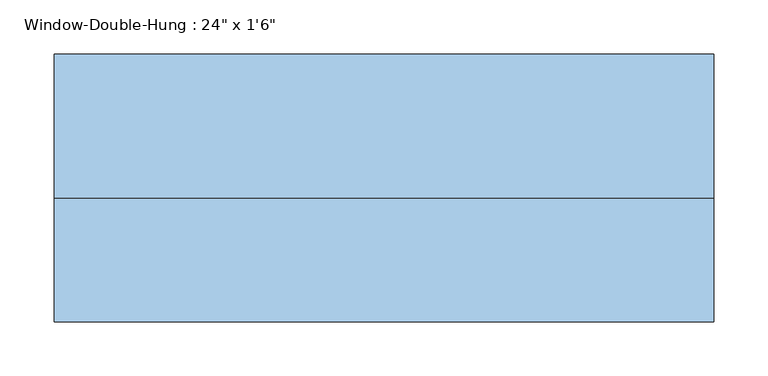
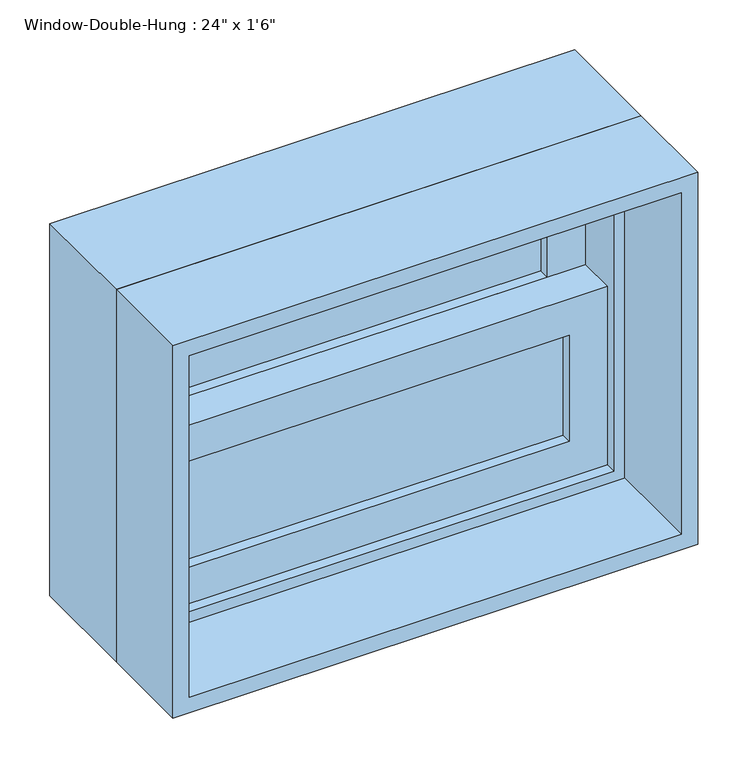
"""IFC4 building model written with IfcOpenShell, lengths in millimetres: window geometry."""

from ifc_helpers import new_model, si_unit, frame, origin, place, context, project, spatial, polyline, outline, extrude, source, transform, mapped, element, save


def window_42222e0e(model_context):
    return source(origin(), model_context, "Body", "SweptSolid", [
        extrude(outline(polyline([(228.6, 44.45), (228.6, 38.1), (-228.6, 38.1), (-228.6, 44.45), (228.6, 44.45)])), frame((0.0, 0.0, 990.6), z_axis=(0.0, 0.0, 1.0), x_axis=(1.0, 0.0, 0.0)), (0.0, 0.0, 1.0), 130.175),
        extrude(outline(polyline([(-228.6, 31.75), (228.6, 31.75), (228.6, 25.4), (-228.6, 25.4), (-228.6, 31.75)])), frame((0.0, 0.0, 990.6), z_axis=(0.0, 0.0, 1.0), x_axis=(1.0, 0.0, 0.0)), (0.0, 0.0, 1.0), 130.175),
        extrude(outline(polyline([(228.6, 88.9), (228.6, 82.55), (-228.6, 82.55), (-228.6, 88.9), (228.6, 88.9)])), frame((0.0, 0.0, 1165.225), z_axis=(0.0, 0.0, 1.0), x_axis=(1.0, 0.0, 0.0)), (0.0, 0.0, 1.0), 130.175),
        extrude(outline(polyline([(-228.6, 76.2), (228.6, 76.2), (228.6, 69.85), (-228.6, 69.85), (-228.6, 76.2)])), frame((0.0, 0.0, 1165.225), z_axis=(0.0, 0.0, 1.0), x_axis=(1.0, 0.0, 0.0)), (0.0, 0.0, 1.0), 130.175),
        extrude(outline(polyline([(1165.225, -273.05), (946.15, -273.05), (946.15, 273.05), (1165.225, 273.05), (1165.225, -273.05)]), holes=[polyline([(1120.775, 228.6), (990.6, 228.6), (990.6, -228.6), (1120.775, -228.6), (1120.775, 228.6)])]), frame((0.0, 12.7, 0.0), z_axis=(0.0, 1.0, 0.0), x_axis=(0.0, 0.0, 1.0)), (0.0, 0.0, 1.0), 44.45),
        extrude(outline(polyline([(1339.85, -273.05), (1120.775, -273.05), (1120.775, 273.05), (1339.85, 273.05), (1339.85, -273.05)]), holes=[polyline([(1295.4, 228.6), (1165.225, 228.6), (1165.225, -228.6), (1295.4, -228.6), (1295.4, 228.6)])]), frame((0.0, 57.15, 0.0), z_axis=(0.0, 1.0, 0.0), x_axis=(0.0, 0.0, 1.0)), (0.0, 0.0, 1.0), 44.45),
        extrude(outline(polyline([(1371.6, -304.8), (914.4, -304.8), (914.4, 304.8), (1371.6, 304.8), (1371.6, -304.8)]), holes=[polyline([(1339.85, 273.05), (946.15, 273.05), (946.15, -273.05), (1339.85, -273.05), (1339.85, 273.05)])]), frame((0.0, 0.0, 0.0), z_axis=(0.0, 1.0, 0.0), x_axis=(0.0, 0.0, 1.0)), (0.0, 0.0, 1.0), 133.35),
        extrude(outline(polyline([(1371.6, 304.8), (1371.6, -304.8), (914.4, -304.8), (914.4, 304.8), (1371.6, 304.8)]), holes=[polyline([(1352.55, 285.75), (933.45, 285.75), (933.45, -285.75), (1352.55, -285.75), (1352.55, 285.75)])]), frame((0.0, -114.3, 0.0), z_axis=(0.0, 1.0, 0.0), x_axis=(0.0, 0.0, 1.0)), (0.0, 0.0, 1.0), 114.3),
    ])


if __name__ == "__main__":
    model = new_model("IFC4")
    model_context = context("Model", 3, world=origin())
    ifc_project = project(units=[si_unit("LENGTHUNIT", "METRE", prefix="MILLI")], contexts=[model_context])
    site = spatial("IfcSite", under=ifc_project)
    building = spatial("IfcBuilding", under=site)
    placement = place(None, origin())
    window_shape = window_42222e0e(model_context)
    element("IfcWindow", 1, ObjectType="Window-Double-Hung : 24\" x 1'6\"", at=placement, inside=building, context=model_context, shape_type="MappedRepresentation", body=[
        mapped(window_shape, transform((0.0, 0.0, 0.0), x_axis=(1.0, 0.0, 0.0), y_axis=(0.0, 1.0, 0.0), z_axis=(0.0, 0.0, 1.0))),
    ])
    save(model, "model.ifc")

# Revit data of these elements
# Type "Window-Double-Hung : 24\" x 1'6\""
#   Type Mark = "19"
#   Fire Rating = "0.5h"
#   Construction Type Id = "DG-DR"
#   Assembly Code = "B2020100"
#   Analytic Construction = "Double glazing - domestic"
#   Wall Thickness [instance default] = 0' - 6"
#   Window Inset [instance default] = 0' - 0"
#   Visual Light Transmittance = 0.81
#   Thermal Resistance (R) = 1.8146 (h·ft²·°F)/BTU
#   Solar Heat Gain Coefficient = 0.76
#   Muntin Width = 1' - 6"
#   Muntin Height = 0' - 5 1/8"
#   Interior Wall Closure [instance default] = 0' - 1 1/2"
#   Rough Width = 2' - 0 1/2"
#   Rough Height = 1' - 6 1/2"
#   Frame Extension [instance default] = 0' - 1 1/4"
#   Exterior Wall Closure [instance default] = 0' - 0 1/2"
#   Extension Jamb [instance default] = 0' - 1 1/2"
#   Heat Transfer Coefficient (U) = 0.5511 BTU/(h·ft²·°F)
#   Height = 1' - 6"
#   Width = 2' - 0"
#   Top Muntin Visibility = yes
#   Indicator Visibility [instance default] = yes
#   Extension Jamb Visibility [instance default] = yes
#   Interior Trim Visibility [instance default] = yes
#   Exterior Trim Visibility [instance default] = yes
#   Define Thermal Properties by = 1
#   Bottom Muntin Visibility = yes
#   Muntin Pattern = Muntin Pattern_2x2 : Muntin Pattern_2x2
#   Interior Trim Material = Wood - Stained
#   Interior Trim = Trim-Window-Interior-Flat : Picture Frame
#   Exterior Trim Material = Clad - White
#   Exterior Trim = Trim-Window-Exterior-Flat : with Sill
#   Glass Panel Material = Glass
#   Exterior Frame Material = Clad - White
#   Interior Frame Material = Wood - Stained
#   Wall Closure = (empty or 0)
# Element 1 (IfcWindow, "Window-Double-Hung : 24\" x 1'6\"")
#   Wall Thickness = 0' - 9"
#   Extension Jamb = 0' - 4 1/2"
#   Materials on its faces: "Wood - Stained", "Glass", "Clad - White"
# Materials
#   "Wood - Stained": class "Wood", colour RGB 224 178 126, transparency 0, Cost = 0
#   "Clad - White": class "Wood", colour RGB 242 242 238, transparency 0, Cost = 0
#   "Glass": class "Glass", colour RGB 0 128 192, transparency 0.75, Description = "Soda Lime Glass", Cost = 0
